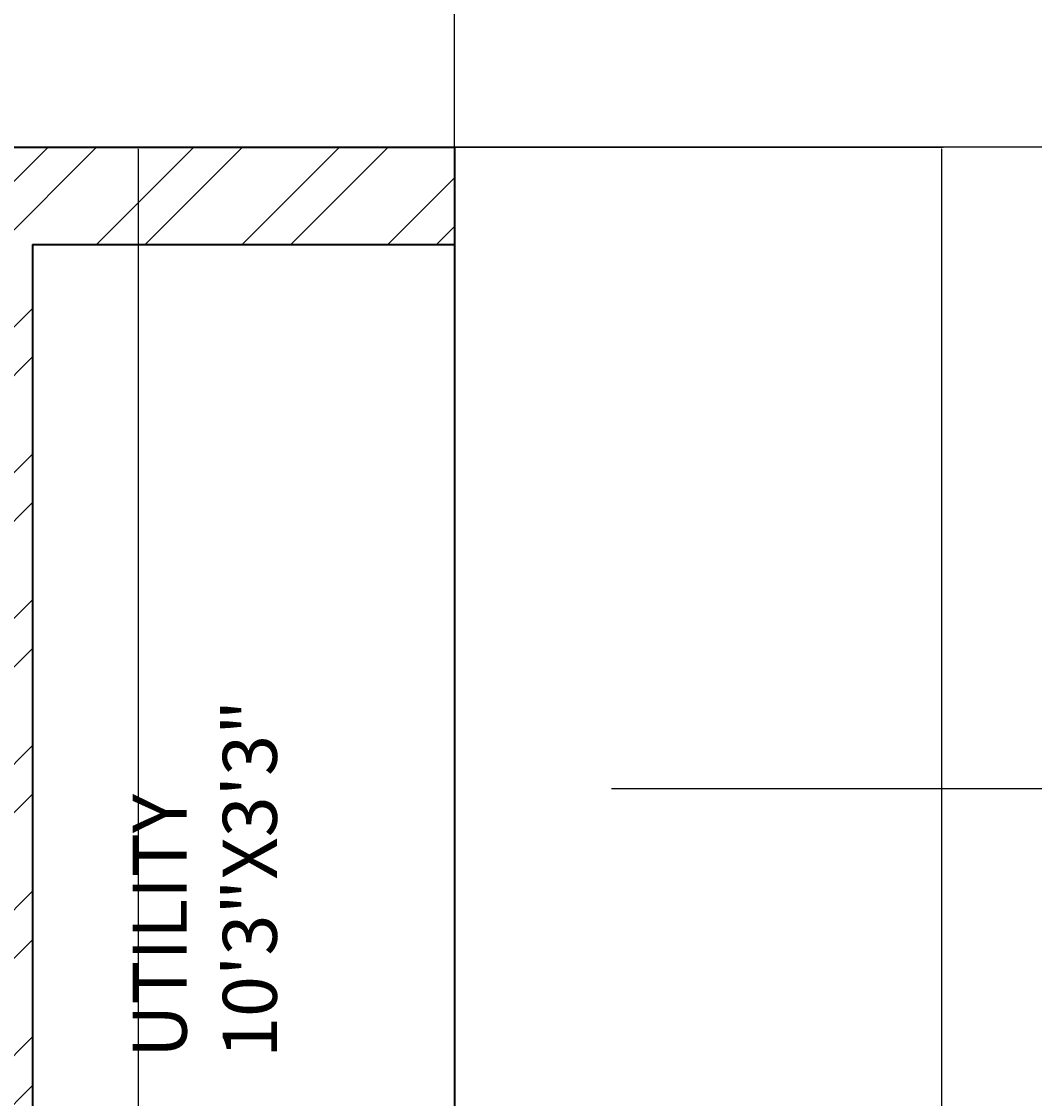
# Model space of a CAD drawing. Units: inches. Extents: x 2120 to 4013, y 1390 to 3019.
# Tile 46 of 59: x 2970 to 3063, y 2265 to 2364. Entities that reach past the tile are written whole.
import ezdxf

# ---------------------------------------------------------------- set-up
doc = ezdxf.new("R2010")
doc.units = ezdxf.units.IN
for name, color, linetype, lineweight in [('A-ANNO-DIMS', 2, 'Continuous', 18), ('A-ANNO-SYMB', 2, 'Continuous', 25), ('A-AREA-IDEN', 7, 'Continuous', 18), ('A-WALL', 7, 'Continuous', 35), ('A-WALL-PATT', 252, 'Continuous', 13)]:
    doc.layers.add(name, color=color, linetype=linetype, lineweight=lineweight)
doc.styles.get("Standard").update_dxf_attribs({"font": 'arial.ttf'})
doc.dimstyles.get("Standard").update_dxf_attribs({"dimtxt": 0.18, "dimasz": 0.18, "dimexe": 0.18, "dimexo": 0.0625, "dimgap": 0.09, "dimtad": 0, "dimtih": 1, "dimtoh": 1, "dimdec": 4, "dimzin": 0, "dimdsep": 46, "dimtxsty": 'Standard', "dimcen": 0.09, "dimadec": 0, "dimazin": 0, "dimtfac": 1, "dimtdec": 4, "dimtofl": 0, "dimtmove": 0, "dimatfit": 3, "dimfxl": 1, "dimtolj": 1, "dimtzin": 0, "dimarcsym": 0})

# ---------------------------------------------------------------- blocks, each defined once
blk = doc.blocks.new('*D211')
at = {"layer": 'A-ANNO-DIMS', "color": 0, "lineweight": -2, "transparency": 16777216}
for p, q in [((2262.733, 2352.593), (2262.733, 2397.711)), ((2262.913, 2397.531), (2635.945, 2397.531)), ((3009.553, 2397.531), (2636.521, 2397.531)), ((3009.733, 2352.593), (3009.733, 2397.711))]:
    blk.add_line(p, q, dxfattribs=at)
at = {"layer": 'A-ANNO-DIMS', "color": 0, "transparency": 16777216}
for points in [[(2262.913, 2397.561), (2262.913, 2397.501), (2262.733, 2397.531)], [(3009.553, 2397.561), (3009.553, 2397.501), (3009.733, 2397.531)]]:
    blk.add_solid(points, dxfattribs=at)
at = {"layer": 'Defpoints', "color": 0, "transparency": 16777216}
for p in [(3009.733, 2397.531), (2262.733, 2352.531), (3009.733, 2352.531)]:
    blk.add_point(p, dxfattribs=at)
at = {"layer": 'A-ANNO-DIMS', "color": 0, "transparency": 16777216, "insert": (2636.233, 2397.531), "char_height": 0.18, "attachment_point": 5}
blk.add_mtext('\\A1;747', dxfattribs=at)
blk = doc.blocks.new('*D212')
at = {"layer": 'A-ANNO-DIMS', "color": 0, "lineweight": -2, "transparency": 16777216}
for p, q in [((3009.796, 2352.531), (3054.913, 2352.531)), ((3054.733, 2352.351), (3054.733, 1947.713)), ((3054.733, 1542.711), (3054.733, 1947.349)), ((3009.796, 1542.531), (3054.913, 1542.531))]:
    blk.add_line(p, q, dxfattribs=at)
at = {"layer": 'A-ANNO-DIMS', "color": 0, "transparency": 16777216}
for points in [[(3054.703, 2352.351), (3054.763, 2352.351), (3054.733, 2352.531)], [(3054.703, 1542.711), (3054.763, 1542.711), (3054.733, 1542.531)]]:
    blk.add_solid(points, dxfattribs=at)
at = {"layer": 'Defpoints', "color": 0, "transparency": 16777216}
for p in [(3009.733, 2352.531), (3009.733, 1542.531), (3054.733, 1542.531)]:
    blk.add_point(p, dxfattribs=at)
at = {"layer": 'A-ANNO-DIMS', "color": 0, "transparency": 16777216, "insert": (3054.733, 1947.531), "char_height": 0.18, "attachment_point": 5}
blk.add_mtext('\\A1;810', dxfattribs=at)
blk = doc.blocks.new('*D217')
at = {"layer": 'A-ANNO-DIMS', "color": 0, "lineweight": -2, "transparency": 16777216}
for p, q in [((3071.672, 2352.531), (2980.308, 2352.531)), ((2980.488, 2352.351), (2980.488, 1947.713)), ((2980.488, 1542.711), (2980.488, 1947.349)), ((3305.672, 1542.531), (2980.308, 1542.531))]:
    blk.add_line(p, q, dxfattribs=at)
at = {"layer": 'A-ANNO-DIMS', "color": 0, "transparency": 16777216}
for points in [[(2980.458, 2352.351), (2980.518, 2352.351), (2980.488, 2352.531)], [(2980.458, 1542.711), (2980.518, 1542.711), (2980.488, 1542.531)]]:
    blk.add_solid(points, dxfattribs=at)
at = {"layer": 'Defpoints', "color": 0, "transparency": 16777216}
for p in [(2980.488, 2352.531), (3071.735, 2352.531), (3305.735, 1542.531)]:
    blk.add_point(p, dxfattribs=at)
at = {"layer": 'A-ANNO-DIMS', "color": 0, "transparency": 16777216, "insert": (2980.488, 1947.531), "char_height": 0.18, "attachment_point": 5}
blk.add_mtext('\\A1;810', dxfattribs=at)

msp = doc.modelspace()

# ---------------------------------------------------------------- hatches: boundary and pattern name
at = {"layer": 'A-WALL-PATT'}
h = msp.add_hatch(dxfattribs=at)
h.set_pattern_fill('ANSI32', color=256)
h.paths.add_polyline_path([(2271.7331, 2343.531), (2283.3788, 2343.531), (2283.3788, 2348.031), (2283.3788, 2352.5306), (2262.7331, 2352.5306), (2262.7331, 2182.638), (2267.2331, 2182.638), (2271.7331, 2182.638), (2271.7331, 2219.031), (2391.7331, 2219.031), (2391.7331, 2214.189), (2393.9831, 2214.189), (2396.2331, 2214.189), (2396.2331, 2219.031), (2420.2331, 2219.031), (2420.2331, 2225.7535), (2417.2197, 2225.7535), (2415.7331, 2225.7535), (2415.7331, 2223.5306), (2271.7331, 2223.5306)])
h.paths.add_polyline_path([(2380.0942, 2352.5306), (2343.3788, 2352.5306), (2343.3788, 2343.531), (2363.2331, 2343.531), (2363.2331, 2288.8489), (2365.4831, 2288.8489), (2367.7331, 2288.8489), (2367.7331, 2343.531), (2380.0942, 2343.531)], flags=17)
h.paths.add_polyline_path([(2432.4339, 2352.5306), (2404.0943, 2352.5306), (2404.0943, 2343.531), (2415.7331, 2343.531), (2415.7331, 2264.0306), (2367.7331, 2264.0306), (2367.7331, 2266.4872), (2363.2331, 2266.4872), (2363.2331, 2259.531), (2367.7331, 2259.531), (2415.7331, 2259.531), (2415.7331, 2255.0658), (2420.2331, 2255.0658), (2420.2331, 2259.531), (2424.5717, 2259.531), (2424.5717, 2261.781), (2424.5717, 2264.0306), (2420.2331, 2264.0306), (2420.2331, 2343.531), (2432.4339, 2343.531)])
h.paths.add_polyline_path([(2508.9115, 2352.5306), (2456.4339, 2352.5306), (2456.4339, 2343.531), (2468.2331, 2343.531), (2468.2331, 2264.0306), (2448.0487, 2264.0306), (2448.0487, 2259.531), (2468.2331, 2259.531), (2468.2331, 2255.5496), (2472.7331, 2255.5496), (2472.7331, 2343.531), (2508.9115, 2343.531)])
h.paths.add_polyline_path([(2637.7331, 2352.5306), (2544.9116, 2352.5306), (2544.9116, 2343.531), (2589.7331, 2343.531), (2633.2331, 2343.531), (2637.7331, 2343.531)])
h.paths.add_polyline_path([(2594.2331, 2343.5306), (2589.7331, 2343.5306), (2589.7331, 2259.5306), (2589.7331, 2252.4915), (2591.9831, 2252.4915), (2594.2331, 2252.4915)])
h.paths.add_polyline_path([(2637.7331, 2223.5306), (2594.2331, 2223.5306), (2594.2331, 2230.1988), (2591.9831, 2230.1988), (2589.7331, 2230.1988), (2589.7331, 2223.5306), (2472.7331, 2223.5306), (2468.2331, 2223.5306), (2468.2331, 2219.031), (2628.7331, 2219.031), (2628.7331, 2138.031), (2637.7331, 2138.031)])
h.paths.add_polyline_path([(3822.6535, 2458.4402), (3874.9468, 2458.4402), (3874.9468, 2476.9866), (3822.6535, 2476.9866)], flags=9)
h.paths.add_polyline_path([(3834.6921, 2781.8174), (3935.9206, 2781.8174), (3935.9206, 2800.3638), (3834.6921, 2800.3638)], flags=9)
h.paths.add_polyline_path([(3832.2843, 2837.9683), (3884.5776, 2837.9683), (3884.5776, 2856.5146), (3832.2843, 2856.5146)], flags=9)
h.paths.add_polyline_path([(3830.9388, 2861.4782), (3956.8958, 2861.4782), (3956.8958, 2880.0245), (3830.9388, 2880.0245)], flags=9)
h.paths.add_polyline_path([(3870.6966, 2352.5752), (3887.9272, 2352.5752), (3887.9272, 2377.3037), (3870.6966, 2377.3037)], flags=9)
h.paths.add_polyline_path([(3289.2701, 2413.161), (3435.2223, 2413.161), (3435.2223, 2450.2538), (3289.2701, 2450.2538)], flags=9)
h.paths.add_polyline_path([(2487.6944, 2414.3601), (2637.8335, 2414.3601), (2637.8335, 2451.4528), (2487.6944, 2451.4528)], flags=9)
h.paths.add_polyline_path([(2567.3724, 1457.9199), (2815.296, 1457.9199), (2815.296, 1495.0127), (2567.3724, 1495.0127)], flags=9)
h.paths.add_polyline_path([(2655.3825, 2093.2363), (2685.9555, 2093.2363), (2685.9555, 2111.8937), (2655.3825, 2111.8937)], flags=9)
h.paths.add_polyline_path([(2543.9218, 1550.6671), (2587.8406, 1550.6671), (2587.8406, 1569.3244), (2543.9218, 1569.3244)], flags=9)
h.paths.add_polyline_path([(2905.1384, 1543.8113), (2949.0572, 1543.8113), (2949.0572, 1562.4686), (2905.1384, 1562.4686)], flags=9)
h.paths.add_polyline_path([(2736.4118, 1702.4736), (2784.2153, 1702.4736), (2784.2153, 1721.1309), (2736.4118, 1721.1309)], flags=9)
h.paths.add_polyline_path([(2912.8666, 1710.4168), (2951.707, 1710.4168), (2951.707, 1729.0741), (2912.8666, 1729.0741)], flags=9)
h.paths.add_polyline_path([(2923.5785, 1763.5038), (2959.7279, 1763.5038), (2959.7279, 1782.1611), (2923.5785, 1782.1611)], flags=9)
h.paths.add_polyline_path([(2925.2114, 1809.6137), (2967.1861, 1809.6137), (2967.1861, 1828.271), (2925.2114, 1828.271)], flags=9)
h.paths.add_polyline_path([(2996.2711, 1878.9003), (2996.2711, 1913.109), (2977.6138, 1913.109), (2977.6138, 1878.9003)], flags=9)
h.paths.add_polyline_path([(2883.0859, 1895.7192), (2927.1855, 1895.7192), (2927.1855, 1914.3766), (2883.0859, 1914.3766)], flags=9)
h.paths.add_polyline_path([(2787.3924, 1810.8013), (2841.0213, 1810.8013), (2841.0213, 1829.4587), (2787.3924, 1829.4587)], flags=9)
h.paths.add_polyline_path([(2775.6399, 2101.7395), (2829.2689, 2101.7395), (2829.2689, 2120.3968), (2775.6399, 2120.3968)], flags=9)
h.paths.add_polyline_path([(2913.0263, 2075.817), (2951.8667, 2075.817), (2951.8667, 2094.4744), (2913.0263, 2094.4744)], flags=9)
h.paths.add_polyline_path([(2929.966, 2133.3669), (2966.1154, 2133.3669), (2966.1154, 2152.0243), (2929.966, 2152.0243)], flags=9)
h.paths.add_polyline_path([(2932.7502, 2182.6088), (2968.8996, 2182.6088), (2968.8996, 2201.2662), (2932.7502, 2201.2662)], flags=9)
h.paths.add_polyline_path([(2996.0681, 2266.3173), (2996.0681, 2300.5261), (2977.4108, 2300.5261), (2977.4108, 2266.3173)], flags=9)
h.paths.add_polyline_path([(2885.1039, 2279.2186), (2929.2035, 2279.2186), (2929.2035, 2297.8759), (2885.1039, 2297.8759)], flags=9)
h.paths.add_polyline_path([(2735.7042, 2218.3197), (2783.5078, 2218.3197), (2783.5078, 2236.9771), (2735.7042, 2236.9771)], flags=9)
h.paths.add_polyline_path([(2635.6049, 2044.0085), (2648.9678, 2044.0085), (2648.9678, 2054.312), (2635.6049, 2054.312)], flags=9)
h.paths.add_polyline_path([(2714.0148, 1923.0473), (2727.3777, 1923.0473), (2727.3777, 1933.3508), (2714.0148, 1933.3508)], flags=9)
h.paths.add_polyline_path([(2709.0345, 1988.1628), (2722.3974, 1988.1628), (2722.3974, 1998.4663), (2709.0345, 1998.4663)], flags=9)
h.paths.add_polyline_path([(2592.8935, 1962.1763), (2606.2564, 1962.1763), (2606.2564, 1972.4799), (2592.8935, 1972.4799)], flags=9)
h.paths.add_polyline_path([(2618.3996, 1985.9724), (2644.1942, 1985.9724), (2644.1942, 1996.2759), (2618.3996, 1996.2759)], flags=9)
h.paths.add_polyline_path([(2601.279, 1920.5869), (2614.6419, 1920.5869), (2614.6419, 1930.8904), (2601.279, 1930.8904)], flags=9)
h.paths.add_polyline_path([(2692.3278, 1932.7645), (2704.5311, 1932.7645), (2704.5311, 1943.0681), (2692.3278, 1943.0681)], flags=9)
h.paths.add_polyline_path([(2311.122, 1672.7318), (2355.0408, 1672.7318), (2355.0408, 1691.3892), (2311.122, 1691.3892)], flags=9)
h.paths.add_polyline_path([(2456.2551, 1632.3198), (2492.4796, 1632.3198), (2492.4796, 1650.9772), (2456.2551, 1650.9772)], flags=9)
h.paths.add_polyline_path([(2401.0766, 1631.4793), (2437.301, 1631.4793), (2437.301, 1650.1367), (2401.0766, 1650.1367)], flags=9)
h.paths.add_polyline_path([(2546.7054, 1700.9235), (2594.509, 1700.9235), (2594.509, 1719.5809), (2546.7054, 1719.5809)], flags=9)
h.paths.add_polyline_path([(2445.4866, 1766.9937), (2497.5261, 1766.9937), (2497.5261, 1785.651), (2445.4866, 1785.651)], flags=9)
h.paths.add_polyline_path([(2287.9992, 1739.7675), (2326.8396, 1739.7675), (2326.8396, 1758.4248), (2287.9992, 1758.4248)], flags=9)
h.paths.add_polyline_path([(2458.5279, 1924.7607), (2510.5675, 1924.7607), (2510.5675, 1943.4181), (2458.5279, 1943.4181)], flags=9)
h.paths.add_polyline_path([(2309.2811, 1902.7642), (2345.4305, 1902.7642), (2345.4305, 1921.4215), (2309.2811, 1921.4215)], flags=9)
h.paths.add_polyline_path([(2490.7554, 2018.9392), (2530.7896, 2018.9392), (2530.7896, 2037.5965), (2490.7554, 2037.5965)], flags=9)
h.paths.add_polyline_path([(2402.143, 2024.7393), (2438.5414, 2024.7393), (2438.5414, 2043.3966), (2402.143, 2043.3966)], flags=9)
h.paths.add_polyline_path([(2287.856, 1931.7926), (2326.6964, 1931.7926), (2326.6964, 1950.4499), (2287.856, 1950.4499)], flags=9)
h.paths.add_polyline_path([(2281.7979, 2193.5771), (2320.6383, 2193.5771), (2320.6383, 2212.2344), (2281.7979, 2212.2344)], flags=25)
h.paths.add_polyline_path([(2484.0754, 2093.892), (2536.115, 2093.892), (2536.115, 2112.5494), (2484.0754, 2112.5494)], flags=9)
h.paths.add_polyline_path([(2624.7948, 2281.8639), (2624.7948, 2311.4137), (2606.1375, 2311.4137), (2606.1375, 2281.8639)], flags=9)
h.paths.add_polyline_path([(2507.5036, 2290.3639), (2541.934, 2290.3639), (2541.934, 2309.0212), (2507.5036, 2309.0212)], flags=9)
h.paths.add_polyline_path([(2423.1076, 2285.2202), (2459.332, 2285.2202), (2459.332, 2303.8776), (2423.1076, 2303.8776)], flags=9)
h.paths.add_polyline_path([(2374.5467, 2289.6272), (2410.7711, 2289.6272), (2410.7711, 2308.2846), (2374.5467, 2308.2846)], flags=25)
h.paths.add_polyline_path([(2277.4907, 2227.5651), (2316.3311, 2227.5651), (2316.3311, 2246.2224), (2277.4907, 2246.2224)], flags=25)
h.paths.add_polyline_path([(2655.3825, 2093.2367), (2685.9555, 2093.2367), (2685.9555, 2111.894), (2655.3825, 2111.894)], flags=9)
h.paths.add_polyline_path([(2543.9217, 1550.6674), (2587.8406, 1550.6674), (2587.8406, 1569.3247), (2543.9217, 1569.3247)], flags=9)
h.paths.add_polyline_path([(2905.1384, 1543.8116), (2949.0572, 1543.8116), (2949.0572, 1562.4689), (2905.1384, 1562.4689)], flags=9)
h.paths.add_polyline_path([(2736.4118, 1702.4739), (2784.2153, 1702.4739), (2784.2153, 1721.1312), (2736.4118, 1721.1312)], flags=9)
h.paths.add_polyline_path([(2912.8666, 1710.4171), (2951.707, 1710.4171), (2951.707, 1729.0744), (2912.8666, 1729.0744)], flags=9)
h.paths.add_polyline_path([(2923.5785, 1763.5041), (2959.7279, 1763.5041), (2959.7279, 1782.1614), (2923.5785, 1782.1614)], flags=9)
h.paths.add_polyline_path([(2925.2114, 1809.614), (2967.1861, 1809.614), (2967.1861, 1828.2713), (2925.2114, 1828.2713)], flags=9)
h.paths.add_polyline_path([(2996.2711, 1878.9006), (2996.2711, 1913.1094), (2977.6137, 1913.1094), (2977.6137, 1878.9006)], flags=9)
h.paths.add_polyline_path([(2883.0859, 1895.7195), (2927.1855, 1895.7195), (2927.1855, 1914.3769), (2883.0859, 1914.3769)], flags=9)
h.paths.add_polyline_path([(2787.3924, 1810.8016), (2841.0213, 1810.8016), (2841.0213, 1829.459), (2787.3924, 1829.459)], flags=9)
h.paths.add_polyline_path([(2775.6399, 2101.7398), (2829.2688, 2101.7398), (2829.2688, 2120.3971), (2775.6399, 2120.3971)], flags=9)
h.paths.add_polyline_path([(2913.0263, 2075.8173), (2951.8667, 2075.8173), (2951.8667, 2094.4747), (2913.0263, 2094.4747)], flags=9)
h.paths.add_polyline_path([(2929.966, 2133.3672), (2966.1154, 2133.3672), (2966.1154, 2152.0246), (2929.966, 2152.0246)], flags=9)
h.paths.add_polyline_path([(2932.7502, 2182.6091), (2968.8996, 2182.6091), (2968.8996, 2201.2665), (2932.7502, 2201.2665)], flags=9)
h.paths.add_polyline_path([(2996.0681, 2266.3176), (2996.0681, 2300.5264), (2977.4108, 2300.5264), (2977.4108, 2266.3176)], flags=9)
h.paths.add_polyline_path([(2885.1039, 2279.2189), (2929.2035, 2279.2189), (2929.2035, 2297.8762), (2885.1039, 2297.8762)], flags=9)
h.paths.add_polyline_path([(2735.7042, 2218.32), (2783.5078, 2218.32), (2783.5078, 2236.9774), (2735.7042, 2236.9774)], flags=9)
h.paths.add_polyline_path([(2635.6048, 2044.0088), (2648.9677, 2044.0088), (2648.9677, 2054.3123), (2635.6048, 2054.3123)], flags=9)
h.paths.add_polyline_path([(2714.0148, 1923.0476), (2727.3777, 1923.0476), (2727.3777, 1933.3511), (2714.0148, 1933.3511)], flags=9)
h.paths.add_polyline_path([(2709.0345, 1988.1631), (2722.3974, 1988.1631), (2722.3974, 1998.4666), (2709.0345, 1998.4666)], flags=9)
h.paths.add_polyline_path([(2592.8935, 1962.1766), (2606.2564, 1962.1766), (2606.2564, 1972.4802), (2592.8935, 1972.4802)], flags=9)
h.paths.add_polyline_path([(2618.3995, 1985.9727), (2644.1942, 1985.9727), (2644.1942, 1996.2762), (2618.3995, 1996.2762)], flags=9)
h.paths.add_polyline_path([(2601.279, 1920.5872), (2614.6419, 1920.5872), (2614.6419, 1930.8908), (2601.279, 1930.8908)], flags=9)
h.paths.add_polyline_path([(2692.3278, 1932.7648), (2704.5311, 1932.7648), (2704.5311, 1943.0684), (2692.3278, 1943.0684)], flags=9)
h.paths.add_polyline_path([(2311.122, 1672.7321), (2355.0408, 1672.7321), (2355.0408, 1691.3895), (2311.122, 1691.3895)], flags=9)
h.paths.add_polyline_path([(2456.2551, 1632.3201), (2492.4795, 1632.3201), (2492.4795, 1650.9775), (2456.2551, 1650.9775)], flags=9)
h.paths.add_polyline_path([(2401.0766, 1631.4796), (2437.301, 1631.4796), (2437.301, 1650.137), (2401.0766, 1650.137)], flags=9)
h.paths.add_polyline_path([(2546.7054, 1700.9238), (2594.509, 1700.9238), (2594.509, 1719.5812), (2546.7054, 1719.5812)], flags=9)
h.paths.add_polyline_path([(2445.4866, 1766.994), (2497.5261, 1766.994), (2497.5261, 1785.6513), (2445.4866, 1785.6513)], flags=9)
h.paths.add_polyline_path([(2287.9992, 1739.7678), (2326.8396, 1739.7678), (2326.8396, 1758.4251), (2287.9992, 1758.4251)], flags=9)
h.paths.add_polyline_path([(2458.5279, 1924.7611), (2510.5675, 1924.7611), (2510.5675, 1943.4184), (2458.5279, 1943.4184)], flags=9)
h.paths.add_polyline_path([(2309.2811, 1902.7645), (2345.4305, 1902.7645), (2345.4305, 1921.4218), (2309.2811, 1921.4218)], flags=9)
h.paths.add_polyline_path([(2490.7554, 2018.9395), (2530.7895, 2018.9395), (2530.7895, 2037.5968), (2490.7554, 2037.5968)], flags=9)
h.paths.add_polyline_path([(2402.143, 2024.7396), (2438.5413, 2024.7396), (2438.5413, 2043.3969), (2402.143, 2043.3969)], flags=9)
h.paths.add_polyline_path([(2287.856, 1931.7929), (2326.6964, 1931.7929), (2326.6964, 1950.4502), (2287.856, 1950.4502)], flags=9)
h.paths.add_polyline_path([(2281.7979, 2193.5774), (2320.6383, 2193.5774), (2320.6383, 2212.2347), (2281.7979, 2212.2347)], flags=25)
h.paths.add_polyline_path([(2484.0754, 2093.8924), (2536.115, 2093.8924), (2536.115, 2112.5497), (2484.0754, 2112.5497)], flags=9)
h.paths.add_polyline_path([(2624.7948, 2281.8642), (2624.7948, 2311.414), (2606.1374, 2311.414), (2606.1374, 2281.8642)], flags=9)
h.paths.add_polyline_path([(2507.5035, 2290.3642), (2541.934, 2290.3642), (2541.934, 2309.0215), (2507.5035, 2309.0215)], flags=9)
h.paths.add_polyline_path([(2423.1075, 2285.2205), (2459.332, 2285.2205), (2459.332, 2303.8779), (2423.1075, 2303.8779)], flags=9)
h.paths.add_polyline_path([(2374.5467, 2289.6275), (2410.7711, 2289.6275), (2410.7711, 2308.2849), (2374.5467, 2308.2849)], flags=25)
h.paths.add_polyline_path([(2277.4907, 2227.5654), (2316.3311, 2227.5654), (2316.3311, 2246.2227), (2277.4907, 2246.2227)], flags=25)
h = msp.add_hatch(dxfattribs=at)
h.set_pattern_fill('ANSI32', color=256)
h.paths.add_polyline_path([(2271.7331, 1980.389), (2262.7331, 1980.389), (2262.7331, 1912.8434), (2267.2331, 1912.8434), (2271.7331, 1912.8434), (2271.7331, 1922.531), (2351.2331, 1922.531), (2351.2331, 1901.4728), (2355.7331, 1901.4728), (2355.7331, 1922.531), (2357.9815, 1922.531), (2357.9815, 1926.5306), (2271.7331, 1926.5306)])
h.paths.add_polyline_path([(2589.2331, 1949.1622), (2584.7331, 1949.1622), (2580.2331, 1949.1622), (2580.2331, 1874.5306), (2355.7331, 1874.5306), (2355.7331, 1880.1922), (2351.2331, 1880.1922), (2351.2331, 1874.5306), (2271.7331, 1874.5306), (2271.7331, 1888.8431), (2262.7331, 1888.8431), (2262.7331, 1842.2909), (2267.2331, 1842.2909), (2271.7331, 1842.2909), (2271.7331, 1865.531), (2415.7331, 1865.531), (2415.7331, 1779.7286), (2420.2331, 1779.7286), (2420.2331, 1865.531), (2589.2331, 1865.531)])
h.paths.add_polyline_path([(2271.7331, 1782.2906), (2262.7331, 1782.2906), (2262.7331, 1711.4639), (2267.2331, 1711.4639), (2271.7331, 1711.4639), (2271.7331, 1738.031), (2420.2331, 1738.031), (2420.2331, 1742.531), (2420.2331, 1747.3376), (2417.9831, 1747.3376), (2415.7331, 1747.3376), (2415.7331, 1742.5306), (2271.7331, 1742.5306)])
h.paths.add_polyline_path([(2271.7331, 1627.031), (2362.3957, 1627.031), (2362.3957, 1629.281), (2362.3957, 1631.5306), (2271.7331, 1631.5306), (2271.7331, 1675.4636), (2262.7331, 1675.4636), (2262.7331, 1581.531), (2405.3032, 1581.531), (2405.3032, 1586.031), (2405.3032, 1590.5306), (2396.2331, 1590.5306), (2396.2331, 1691.4513), (2418.7206, 1691.4513), (2418.7206, 1695.951), (2396.2331, 1695.951), (2391.7331, 1695.951), (2391.7331, 1631.5306), (2386.7425, 1631.5306), (2386.7425, 1629.2806), (2386.7425, 1627.031), (2391.7331, 1627.031), (2391.7331, 1586.1709), (2271.7331, 1586.1709)])
h.paths.add_polyline_path([(2459.6703, 1590.5306), (2429.3032, 1590.5306), (2429.3032, 1581.531), (2459.6703, 1581.531), (2459.6703, 1586.031)])
h.paths.add_polyline_path([(2501.2331, 1590.531), (2501.2331, 1665.0195), (2498.9831, 1665.0195), (2496.7331, 1665.0195), (2496.7331, 1590.5306), (2483.8201, 1590.5306), (2483.8201, 1590.1579), (2483.6704, 1590.1579), (2483.6704, 1581.531), (2505.0196, 1581.531), (2505.0196, 1583.781), (2505.0196, 1586.0306), (2501.2331, 1586.0306)])
h.paths.add_polyline_path([(2544.1361, 1583.781), (2544.1361, 1586.0306), (2527.1368, 1586.0306), (2527.1368, 1583.7806), (2527.1368, 1581.531), (2544.1361, 1581.531)])
h.paths.add_polyline_path([(3822.6535, 2458.4402), (3874.9468, 2458.4402), (3874.9468, 2476.9866), (3822.6535, 2476.9866)], flags=9)
h.paths.add_polyline_path([(3834.6921, 2781.8174), (3935.9206, 2781.8174), (3935.9206, 2800.3638), (3834.6921, 2800.3638)], flags=9)
h.paths.add_polyline_path([(3832.2843, 2837.9683), (3884.5776, 2837.9683), (3884.5776, 2856.5146), (3832.2843, 2856.5146)], flags=9)
h.paths.add_polyline_path([(3830.9388, 2861.4782), (3956.8958, 2861.4782), (3956.8958, 2880.0245), (3830.9388, 2880.0245)], flags=9)
h.paths.add_polyline_path([(3870.6966, 2352.5752), (3887.9272, 2352.5752), (3887.9272, 2377.3037), (3870.6966, 2377.3037)], flags=9)
h.paths.add_polyline_path([(3289.2701, 2413.161), (3435.2223, 2413.161), (3435.2223, 2450.2538), (3289.2701, 2450.2538)], flags=9)
h.paths.add_polyline_path([(2487.6944, 2414.3601), (2637.8335, 2414.3601), (2637.8335, 2451.4528), (2487.6944, 2451.4528)], flags=9)
h.paths.add_polyline_path([(2567.3724, 1457.9199), (2815.296, 1457.9199), (2815.296, 1495.0127), (2567.3724, 1495.0127)], flags=9)
h.paths.add_polyline_path([(2655.3825, 2093.2363), (2685.9555, 2093.2363), (2685.9555, 2111.8937), (2655.3825, 2111.8937)], flags=9)
h.paths.add_polyline_path([(2543.9218, 1550.6671), (2587.8406, 1550.6671), (2587.8406, 1569.3244), (2543.9218, 1569.3244)], flags=9)
h.paths.add_polyline_path([(2905.1384, 1543.8113), (2949.0572, 1543.8113), (2949.0572, 1562.4686), (2905.1384, 1562.4686)], flags=9)
h.paths.add_polyline_path([(2736.4118, 1702.4736), (2784.2153, 1702.4736), (2784.2153, 1721.1309), (2736.4118, 1721.1309)], flags=9)
h.paths.add_polyline_path([(2912.8666, 1710.4168), (2951.707, 1710.4168), (2951.707, 1729.0741), (2912.8666, 1729.0741)], flags=9)
h.paths.add_polyline_path([(2923.5785, 1763.5038), (2959.7279, 1763.5038), (2959.7279, 1782.1611), (2923.5785, 1782.1611)], flags=9)
h.paths.add_polyline_path([(2925.2114, 1809.6137), (2967.1861, 1809.6137), (2967.1861, 1828.271), (2925.2114, 1828.271)], flags=9)
h.paths.add_polyline_path([(2996.2711, 1878.9003), (2996.2711, 1913.109), (2977.6138, 1913.109), (2977.6138, 1878.9003)], flags=9)
h.paths.add_polyline_path([(2883.0859, 1895.7192), (2927.1855, 1895.7192), (2927.1855, 1914.3766), (2883.0859, 1914.3766)], flags=9)
h.paths.add_polyline_path([(2787.3924, 1810.8013), (2841.0213, 1810.8013), (2841.0213, 1829.4587), (2787.3924, 1829.4587)], flags=9)
h.paths.add_polyline_path([(2775.6399, 2101.7395), (2829.2689, 2101.7395), (2829.2689, 2120.3968), (2775.6399, 2120.3968)], flags=9)
h.paths.add_polyline_path([(2913.0263, 2075.817), (2951.8667, 2075.817), (2951.8667, 2094.4744), (2913.0263, 2094.4744)], flags=9)
h.paths.add_polyline_path([(2929.966, 2133.3669), (2966.1154, 2133.3669), (2966.1154, 2152.0243), (2929.966, 2152.0243)], flags=9)
h.paths.add_polyline_path([(2932.7502, 2182.6088), (2968.8996, 2182.6088), (2968.8996, 2201.2662), (2932.7502, 2201.2662)], flags=9)
h.paths.add_polyline_path([(2996.0681, 2266.3173), (2996.0681, 2300.5261), (2977.4108, 2300.5261), (2977.4108, 2266.3173)], flags=9)
h.paths.add_polyline_path([(2885.1039, 2279.2186), (2929.2035, 2279.2186), (2929.2035, 2297.8759), (2885.1039, 2297.8759)], flags=9)
h.paths.add_polyline_path([(2735.7042, 2218.3197), (2783.5078, 2218.3197), (2783.5078, 2236.9771), (2735.7042, 2236.9771)], flags=9)
h.paths.add_polyline_path([(2635.6049, 2044.0085), (2648.9678, 2044.0085), (2648.9678, 2054.312), (2635.6049, 2054.312)], flags=9)
h.paths.add_polyline_path([(2714.0148, 1923.0473), (2727.3777, 1923.0473), (2727.3777, 1933.3508), (2714.0148, 1933.3508)], flags=9)
h.paths.add_polyline_path([(2709.0345, 1988.1628), (2722.3974, 1988.1628), (2722.3974, 1998.4663), (2709.0345, 1998.4663)], flags=9)
h.paths.add_polyline_path([(2592.8935, 1962.1763), (2606.2564, 1962.1763), (2606.2564, 1972.4799), (2592.8935, 1972.4799)], flags=9)
h.paths.add_polyline_path([(2618.3996, 1985.9724), (2644.1942, 1985.9724), (2644.1942, 1996.2759), (2618.3996, 1996.2759)], flags=9)
h.paths.add_polyline_path([(2601.279, 1920.5869), (2614.6419, 1920.5869), (2614.6419, 1930.8904), (2601.279, 1930.8904)], flags=9)
h.paths.add_polyline_path([(2692.3278, 1932.7645), (2704.5311, 1932.7645), (2704.5311, 1943.0681), (2692.3278, 1943.0681)], flags=9)
h.paths.add_polyline_path([(2311.122, 1672.7318), (2355.0408, 1672.7318), (2355.0408, 1691.3892), (2311.122, 1691.3892)], flags=25)
h.paths.add_polyline_path([(2456.2551, 1632.3198), (2492.4796, 1632.3198), (2492.4796, 1650.9772), (2456.2551, 1650.9772)], flags=9)
h.paths.add_polyline_path([(2401.0766, 1631.4793), (2437.301, 1631.4793), (2437.301, 1650.1367), (2401.0766, 1650.1367)], flags=9)
h.paths.add_polyline_path([(2546.7054, 1700.9235), (2594.509, 1700.9235), (2594.509, 1719.5809), (2546.7054, 1719.5809)], flags=9)
h.paths.add_polyline_path([(2445.4866, 1766.9937), (2497.5261, 1766.9937), (2497.5261, 1785.651), (2445.4866, 1785.651)], flags=9)
h.paths.add_polyline_path([(2287.9992, 1739.7675), (2326.8396, 1739.7675), (2326.8396, 1758.4248), (2287.9992, 1758.4248)], flags=24)
h.paths.add_polyline_path([(2458.5279, 1924.7607), (2510.5675, 1924.7607), (2510.5675, 1943.4181), (2458.5279, 1943.4181)], flags=25)
h.paths.add_polyline_path([(2309.2811, 1902.7642), (2345.4305, 1902.7642), (2345.4305, 1921.4215), (2309.2811, 1921.4215)], flags=25)
h.paths.add_polyline_path([(2490.7554, 2018.9392), (2530.7896, 2018.9392), (2530.7896, 2037.5965), (2490.7554, 2037.5965)], flags=9)
h.paths.add_polyline_path([(2402.143, 2024.7393), (2438.5414, 2024.7393), (2438.5414, 2043.3966), (2402.143, 2043.3966)], flags=9)
h.paths.add_polyline_path([(2287.856, 1931.7926), (2326.6964, 1931.7926), (2326.6964, 1950.4499), (2287.856, 1950.4499)], flags=25)
h.paths.add_polyline_path([(2281.7979, 2193.5771), (2320.6383, 2193.5771), (2320.6383, 2212.2344), (2281.7979, 2212.2344)], flags=9)
h.paths.add_polyline_path([(2484.0754, 2093.892), (2536.115, 2093.892), (2536.115, 2112.5494), (2484.0754, 2112.5494)], flags=9)
h.paths.add_polyline_path([(2624.7948, 2281.8639), (2624.7948, 2311.4137), (2606.1375, 2311.4137), (2606.1375, 2281.8639)], flags=9)
h.paths.add_polyline_path([(2507.5036, 2290.3639), (2541.934, 2290.3639), (2541.934, 2309.0212), (2507.5036, 2309.0212)], flags=9)
h.paths.add_polyline_path([(2423.1076, 2285.2202), (2459.332, 2285.2202), (2459.332, 2303.8776), (2423.1076, 2303.8776)], flags=9)
h.paths.add_polyline_path([(2374.5467, 2289.6272), (2410.7711, 2289.6272), (2410.7711, 2308.2846), (2374.5467, 2308.2846)], flags=9)
h.paths.add_polyline_path([(2277.4907, 2227.5651), (2316.3311, 2227.5651), (2316.3311, 2246.2224), (2277.4907, 2246.2224)], flags=9)
h.paths.add_polyline_path([(2655.3825, 2093.2367), (2685.9555, 2093.2367), (2685.9555, 2111.894), (2655.3825, 2111.894)], flags=9)
h.paths.add_polyline_path([(2543.9217, 1550.6674), (2587.8406, 1550.6674), (2587.8406, 1569.3247), (2543.9217, 1569.3247)], flags=9)
h.paths.add_polyline_path([(2905.1384, 1543.8116), (2949.0572, 1543.8116), (2949.0572, 1562.4689), (2905.1384, 1562.4689)], flags=9)
h.paths.add_polyline_path([(2736.4118, 1702.4739), (2784.2153, 1702.4739), (2784.2153, 1721.1312), (2736.4118, 1721.1312)], flags=9)
h.paths.add_polyline_path([(2912.8666, 1710.4171), (2951.707, 1710.4171), (2951.707, 1729.0744), (2912.8666, 1729.0744)], flags=9)
h.paths.add_polyline_path([(2923.5785, 1763.5041), (2959.7279, 1763.5041), (2959.7279, 1782.1614), (2923.5785, 1782.1614)], flags=9)
h.paths.add_polyline_path([(2925.2114, 1809.614), (2967.1861, 1809.614), (2967.1861, 1828.2713), (2925.2114, 1828.2713)], flags=9)
h.paths.add_polyline_path([(2996.2711, 1878.9006), (2996.2711, 1913.1094), (2977.6137, 1913.1094), (2977.6137, 1878.9006)], flags=9)
h.paths.add_polyline_path([(2883.0859, 1895.7195), (2927.1855, 1895.7195), (2927.1855, 1914.3769), (2883.0859, 1914.3769)], flags=9)
h.paths.add_polyline_path([(2787.3924, 1810.8016), (2841.0213, 1810.8016), (2841.0213, 1829.459), (2787.3924, 1829.459)], flags=9)
h.paths.add_polyline_path([(2775.6399, 2101.7398), (2829.2688, 2101.7398), (2829.2688, 2120.3971), (2775.6399, 2120.3971)], flags=9)
h.paths.add_polyline_path([(2913.0263, 2075.8173), (2951.8667, 2075.8173), (2951.8667, 2094.4747), (2913.0263, 2094.4747)], flags=9)
h.paths.add_polyline_path([(2929.966, 2133.3672), (2966.1154, 2133.3672), (2966.1154, 2152.0246), (2929.966, 2152.0246)], flags=9)
h.paths.add_polyline_path([(2932.7502, 2182.6091), (2968.8996, 2182.6091), (2968.8996, 2201.2665), (2932.7502, 2201.2665)], flags=9)
h.paths.add_polyline_path([(2996.0681, 2266.3176), (2996.0681, 2300.5264), (2977.4108, 2300.5264), (2977.4108, 2266.3176)], flags=9)
h.paths.add_polyline_path([(2885.1039, 2279.2189), (2929.2035, 2279.2189), (2929.2035, 2297.8762), (2885.1039, 2297.8762)], flags=9)
h.paths.add_polyline_path([(2735.7042, 2218.32), (2783.5078, 2218.32), (2783.5078, 2236.9774), (2735.7042, 2236.9774)], flags=9)
h.paths.add_polyline_path([(2635.6048, 2044.0088), (2648.9677, 2044.0088), (2648.9677, 2054.3123), (2635.6048, 2054.3123)], flags=9)
h.paths.add_polyline_path([(2714.0148, 1923.0476), (2727.3777, 1923.0476), (2727.3777, 1933.3511), (2714.0148, 1933.3511)], flags=9)
h.paths.add_polyline_path([(2709.0345, 1988.1631), (2722.3974, 1988.1631), (2722.3974, 1998.4666), (2709.0345, 1998.4666)], flags=9)
h.paths.add_polyline_path([(2592.8935, 1962.1766), (2606.2564, 1962.1766), (2606.2564, 1972.4802), (2592.8935, 1972.4802)], flags=9)
h.paths.add_polyline_path([(2618.3995, 1985.9727), (2644.1942, 1985.9727), (2644.1942, 1996.2762), (2618.3995, 1996.2762)], flags=9)
h.paths.add_polyline_path([(2601.279, 1920.5872), (2614.6419, 1920.5872), (2614.6419, 1930.8908), (2601.279, 1930.8908)], flags=9)
h.paths.add_polyline_path([(2692.3278, 1932.7648), (2704.5311, 1932.7648), (2704.5311, 1943.0684), (2692.3278, 1943.0684)], flags=9)
h.paths.add_polyline_path([(2311.122, 1672.7321), (2355.0408, 1672.7321), (2355.0408, 1691.3895), (2311.122, 1691.3895)], flags=25)
h.paths.add_polyline_path([(2456.2551, 1632.3201), (2492.4795, 1632.3201), (2492.4795, 1650.9775), (2456.2551, 1650.9775)], flags=9)
h.paths.add_polyline_path([(2401.0766, 1631.4796), (2437.301, 1631.4796), (2437.301, 1650.137), (2401.0766, 1650.137)], flags=9)
h.paths.add_polyline_path([(2546.7054, 1700.9238), (2594.509, 1700.9238), (2594.509, 1719.5812), (2546.7054, 1719.5812)], flags=9)
h.paths.add_polyline_path([(2445.4866, 1766.994), (2497.5261, 1766.994), (2497.5261, 1785.6513), (2445.4866, 1785.6513)], flags=9)
h.paths.add_polyline_path([(2287.9992, 1739.7678), (2326.8396, 1739.7678), (2326.8396, 1758.4251), (2287.9992, 1758.4251)], flags=24)
h.paths.add_polyline_path([(2458.5279, 1924.7611), (2510.5675, 1924.7611), (2510.5675, 1943.4184), (2458.5279, 1943.4184)], flags=25)
h.paths.add_polyline_path([(2309.2811, 1902.7645), (2345.4305, 1902.7645), (2345.4305, 1921.4218), (2309.2811, 1921.4218)], flags=25)
h.paths.add_polyline_path([(2490.7554, 2018.9395), (2530.7895, 2018.9395), (2530.7895, 2037.5968), (2490.7554, 2037.5968)], flags=9)
h.paths.add_polyline_path([(2402.143, 2024.7396), (2438.5413, 2024.7396), (2438.5413, 2043.3969), (2402.143, 2043.3969)], flags=9)
h.paths.add_polyline_path([(2287.856, 1931.7929), (2326.6964, 1931.7929), (2326.6964, 1950.4502), (2287.856, 1950.4502)], flags=25)
h.paths.add_polyline_path([(2281.7979, 2193.5774), (2320.6383, 2193.5774), (2320.6383, 2212.2347), (2281.7979, 2212.2347)], flags=9)
h.paths.add_polyline_path([(2484.0754, 2093.8924), (2536.115, 2093.8924), (2536.115, 2112.5497), (2484.0754, 2112.5497)], flags=9)
h.paths.add_polyline_path([(2624.7948, 2281.8642), (2624.7948, 2311.414), (2606.1374, 2311.414), (2606.1374, 2281.8642)], flags=9)
h.paths.add_polyline_path([(2507.5035, 2290.3642), (2541.934, 2290.3642), (2541.934, 2309.0215), (2507.5035, 2309.0215)], flags=9)
h.paths.add_polyline_path([(2423.1075, 2285.2205), (2459.332, 2285.2205), (2459.332, 2303.8779), (2423.1075, 2303.8779)], flags=9)
h.paths.add_polyline_path([(2374.5467, 2289.6275), (2410.7711, 2289.6275), (2410.7711, 2308.2849), (2374.5467, 2308.2849)], flags=9)
h.paths.add_polyline_path([(2277.4907, 2227.5654), (2316.3311, 2227.5654), (2316.3311, 2246.2227), (2277.4907, 2246.2227)], flags=9)
h = msp.add_hatch(dxfattribs=at)
h.set_pattern_fill('ANSI32', color=256)
h.paths.add_polyline_path([(2271.7331, 2122.6377), (2262.7331, 2122.6377), (2262.7331, 2040.3893), (2267.2331, 2040.3893), (2271.7331, 2040.3893), (2271.7331, 2044.8856), (2271.7331, 2070.531), (2391.7331, 2070.531), (2391.7331, 1926.5306), (2388.3993, 1926.5306), (2388.3993, 1922.531), (2395.7331, 1922.531), (2395.7331, 1992.531), (2400.4511, 1992.531), (2400.4511, 1997.0306), (2395.7331, 1997.0306), (2395.7331, 2070.531), (2443.7331, 2070.531), (2443.7331, 2046.1368), (2448.2331, 2046.1368), (2448.2331, 2070.531), (2580.2331, 2070.531), (2580.2331, 1997.0306), (2492.9076, 1997.0306), (2492.9076, 1992.531), (2580.2331, 1992.531), (2580.2331, 1983.9368), (2589.2331, 1983.9368), (2589.2331, 2070.531), (2589.2331, 2075.0306), (2396.2331, 2075.0306), (2396.2331, 2184.3565), (2393.9831, 2184.3565), (2391.7331, 2184.3565), (2391.7331, 2075.0306), (2271.7331, 2075.0306)])
h.paths.add_polyline_path([(2724.7331, 2138.0306), (2628.7331, 2138.0306), (2628.7331, 2070.5306), (2628.7331, 2067.0987), (2633.2331, 2067.0987), (2637.7331, 2067.0987), (2637.7331, 2070.531), (2657.3413, 2070.531), (2657.3413, 2079.5306), (2637.7331, 2079.5306), (2637.7331, 2129.031), (2715.7331, 2129.031), (2715.7331, 2079.5306), (2698.0378, 2079.5306), (2698.0378, 2070.531), (2715.7331, 2070.531), (2715.7331, 2012.1531), (2720.2331, 2012.1531), (2724.7331, 2012.1531)])
h.paths.add_polyline_path([(2724.7331, 2213.031), (2831.3209, 2213.031), (2831.3209, 2215.281), (2831.3209, 2217.5306), (2724.7331, 2217.5306), (2724.7331, 2343.531), (2751.8755, 2343.531), (2751.8755, 2352.5306), (2715.7331, 2352.5306), (2715.7331, 2138.031), (2724.7331, 2138.031)])
h.paths.add_polyline_path([(2902.53, 2352.5306), (2811.8755, 2352.5306), (2811.8755, 2343.531), (2867.2331, 2343.531), (2867.2331, 2217.5306), (2863.6364, 2217.5306), (2863.6364, 2213.031), (2871.7331, 2213.031), (2871.7331, 2217.531), (2871.7331, 2343.531), (2902.53, 2343.531)])
h.paths.add_polyline_path([(3009.7331, 2352.5306), (2938.53, 2352.5306), (2938.53, 2343.531), (2966.2331, 2343.531), (2966.2331, 2242.3281), (2968.4831, 2242.3281), (2970.7331, 2242.3281), (2970.7331, 2343.531), (3009.7331, 2343.531)])
h.paths.add_polyline_path([(3009.7331, 2217.5306), (2970.7331, 2217.5306), (2970.7331, 2220.5422), (2968.4831, 2220.5422), (2966.2331, 2220.5422), (2966.2331, 2217.5306), (2911.7752, 2217.5306), (2907.7331, 2217.5306), (2907.7331, 2213.0306), (2907.7331, 2194.9663), (2912.2331, 2194.9663), (2912.2331, 2213.031), (2970.7331, 2213.031), (3000.7331, 2213.031), (3000.7331, 2205.523), (3009.7331, 2205.523)])
h.paths.add_polyline_path([(3009.7331, 2181.5227), (3000.7331, 2181.5227), (3000.7331, 2165.0306), (2912.2331, 2165.0306), (2912.2331, 2170.8202), (2907.7331, 2170.8202), (2907.7331, 2165.0306), (2899.5169, 2165.0306), (2899.5169, 2162.7806), (2899.5169, 2160.531), (2907.7331, 2160.531), (2907.7331, 2137.3432), (2912.2331, 2137.3432), (2912.2331, 2160.531), (3000.7331, 2160.531), (3000.7331, 2150.4993), (3009.7331, 2150.4993)])
h.paths.add_polyline_path([(3009.7331, 2126.499), (3005.2331, 2126.499), (3000.7331, 2126.499), (3000.7331, 2112.5306), (2912.2331, 2112.5306), (2912.2331, 2115.6036), (2907.7331, 2115.6036), (2907.7331, 2108.031), (3000.7331, 2108.031), (3000.7331, 2084.7256), (3009.7331, 2084.7256)], flags=17)
h.paths.add_polyline_path([(3009.7331, 1971.531), (3009.7331, 2024.7253), (3000.7331, 2024.7253), (3000.7331, 2006.4153), (3000.7331, 1971.5306), (2864.2331, 1971.5306), (2864.2331, 2160.531), (2868.0522, 2160.531), (2868.0522, 2165.0306), (2859.7331, 2165.0306), (2859.7331, 1971.5306), (2724.7331, 1971.5306), (2724.7331, 1977.7012), (2715.7331, 1977.7012), (2715.7331, 1962.5306), (2715.7331, 1950.9035), (2720.2331, 1950.9035), (2724.7331, 1950.9035), (2724.7331, 1962.531), (2855.2331, 1962.531), (2859.7331, 1962.531), (2859.7331, 1835.031), (2864.2331, 1834.8158), (2864.2331, 1962.531), (2958.7331, 1962.531), (2958.7331, 1937.0925), (2963.2331, 1937.0925), (2963.2331, 1962.531), (3000.7331, 1962.531), (3009.7331, 1962.531)])
h.paths.add_polyline_path([(2724.7331, 1728.531), (2822.7164, 1728.531), (2822.7164, 1733.0306), (2724.7331, 1733.0306), (2724.7331, 1779.3416), (2715.7331, 1779.3416), (2715.7331, 1581.531), (2753.02, 1581.531), (2753.02, 1586.031), (2753.02, 1590.5306), (2724.7331, 1590.5306)])
h.paths.add_polyline_path([(2864.2331, 1590.531), (2864.2331, 1787.031), (2868.4075, 1787.031), (2868.4075, 1791.5306), (2859.7331, 1791.5306), (2859.7331, 1739.0306), (2859.7331, 1733.0306), (2854.3125, 1733.0306), (2854.3125, 1728.531), (2859.7331, 1728.531), (2859.7331, 1590.5306), (2813.02, 1590.5306), (2813.02, 1581.531), (2868.4123, 1581.531), (2868.4123, 1583.781), (2868.4123, 1586.0306), (2864.2331, 1586.0306)])
h.paths.add_polyline_path([(3009.7331, 1754.6619), (3000.7331, 1754.6619), (3000.7331, 1739.0306), (2912.2331, 1739.0306), (2912.2331, 1742.2257), (2907.7331, 1742.2257), (2907.7331, 1739.0306), (2907.7331, 1734.531), (3000.7331, 1734.531), (3000.7331, 1590.5306), (3000.7331, 1586.0306), (2971.3921, 1586.0306), (2971.3921, 1581.531), (3009.7331, 1581.531)])
h.paths.add_polyline_path([(2911.3921, 1583.781), (2911.3921, 1586.0306), (2891.2138, 1586.0306), (2891.2138, 1581.531), (2911.3921, 1581.531)])
h.paths.add_polyline_path([(3009.7331, 1799.8422), (3000.7331, 1799.8422), (3000.7331, 1791.5306), (2912.2331, 1791.5306), (2912.2331, 1796.3264), (2909.9831, 1796.3264), (2907.7331, 1796.3264), (2907.7331, 1791.5306), (2902.7033, 1791.5306), (2902.7033, 1787.031), (2907.7331, 1787.031), (2907.7331, 1761.1622), (2912.2331, 1761.1622), (2912.2331, 1787.031), (3000.7331, 1787.031), (3000.7331, 1778.6622), (3009.7331, 1778.6622)])
h.paths.add_polyline_path([(3009.7331, 1839.5306), (2963.2331, 1839.5306), (2963.2331, 1842.8629), (2960.9831, 1842.8629), (2958.7331, 1842.8629), (2958.7331, 1839.5306), (2907.7331, 1839.5306), (2907.7331, 1814.4599), (2912.2331, 1814.4599), (2912.2331, 1835.031), (3000.7331, 1835.031), (3000.7331, 1823.8425), (3009.7331, 1823.8425), (3009.7331, 1835.031)])
h.paths.add_polyline_path([(2963.2331, 1901.0922), (2960.9831, 1901.0922), (2958.7331, 1901.0922), (2958.7331, 1862.8843), (2963.2331, 1862.8843)], flags=17)
h.paths.add_polyline_path([(2724.7331, 1891.9826), (2724.7331, 1914.3416), (2715.7331, 1914.3416), (2715.7331, 1783.8416), (2637.7331, 1783.8416), (2637.7331, 1914.3416), (2628.7331, 1914.3416), (2624.7701, 1914.3416), (2624.7701, 1909.8416), (2624.7701, 1905.3419), (2628.7331, 1905.3419), (2628.7331, 1876.9915), (2628.7331, 1779.3419), (2637.7331, 1779.3419), (2715.7331, 1779.3419), (2724.7331, 1779.3419), (2724.7331, 1835.031)])
h.paths.add_polyline_path([(2637.7331, 1731.531), (2637.7331, 1779.3416), (2628.7331, 1779.3416), (2628.7331, 1731.5306), (2589.2331, 1731.5306), (2535.9814, 1731.5306), (2496.7331, 1731.5306), (2496.7331, 1725.6876), (2498.9831, 1725.6876), (2501.2331, 1725.6876), (2501.2331, 1727.031), (2628.7331, 1727.031), (2628.7331, 1680.4203), (2628.7331, 1590.5306), (2628.7331, 1586.0306), (2604.1361, 1586.0306), (2604.1361, 1581.531), (2637.7331, 1581.531), (2637.7331, 1590.531)])

# ---------------------------------------------------------------- linework, layer by layer
at = {"layer": 'A-ANNO-SYMB'}
msp.add_line((3024.2377, 2293.2324), (3883.8033, 2293.2324), dxfattribs=at)
at = {"layer": 'A-WALL'}
for p, q in [((2715.7331, 2352.531), (3009.7331, 2352.531)), ((2715.7331, 2352.5306), (3009.7331, 2352.5306)), ((3009.7331, 2352.531), (3009.7331, 2075.031)), ((3009.7331, 2352.5306), (3009.7331, 2075.0306)), ((2970.7331, 2343.531), (2970.7331, 2240.8622)), ((2970.7331, 2343.531), (3009.7331, 2343.531)), ((2970.7331, 2343.531), (3009.7331, 2343.531)), ((2970.7331, 2343.5306), (3009.7331, 2343.5306)), ((2970.7331, 2343.5306), (2970.7331, 2240.8619)), ((2970.7331, 2343.5306), (3009.7331, 2343.5306))]:
    msp.add_line(p, q, dxfattribs=at)

# ---------------------------------------------------------------- texts
at = {"layer": 'A-AREA-IDEN', "char_height": 5, "attachment_point": 1, "rotation": 90}
for insert in [(2979.9841, 2268.3282), (2979.9841, 2268.3279)]:
    msp.add_mtext_dynamic_manual_height_columns('UTILITY\\P10\'3"X3\'3"', width=183.84076, gutter_width=12.5, heights=[0], dxfattribs=dict(at, insert=insert))

# ---------------------------------------------------------------- dimensions: what is measured, and where the dimension line sits
at = {"layer": 'A-ANNO-DIMS'}
dim = msp.add_linear_dim(base=(3009.7331, 2397.531), p1=(2262.7331, 2352.531), p2=(3009.7331, 2352.531), dimstyle='Standard', override={"dimdec": 0, "dimlfac": 1, "dimrnd": 0, "dimzin": 0, "dimdsep": 46, "dimlunit": 2}, dxfattribs=at)
dim.commit()
dim.dimension.update_dxf_attribs({"geometry": '*D211', "text_midpoint": (2636.2331, 2397.531)})
for base, p1, p2, picture, middle in [((2980.4877, 2352.531), (3305.7347, 1542.531), (3071.7347, 2352.531), '*D217', (2980.4877, 1947.531)), ((3054.7331, 1542.531), (3009.7331, 2352.531), (3009.7331, 1542.531), '*D212', (3054.7331, 1947.531))]:
    dim = msp.add_linear_dim(base=base, p1=p1, p2=p2, angle=90, dimstyle='Standard', override={"dimdec": 0, "dimlfac": 1, "dimrnd": 0, "dimzin": 0, "dimdsep": 46, "dimlunit": 2}, dxfattribs=at)
    dim.commit()
    dim.dimension.update_dxf_attribs({"geometry": picture, "text_midpoint": middle})

doc.saveas('drawing.dxf')
